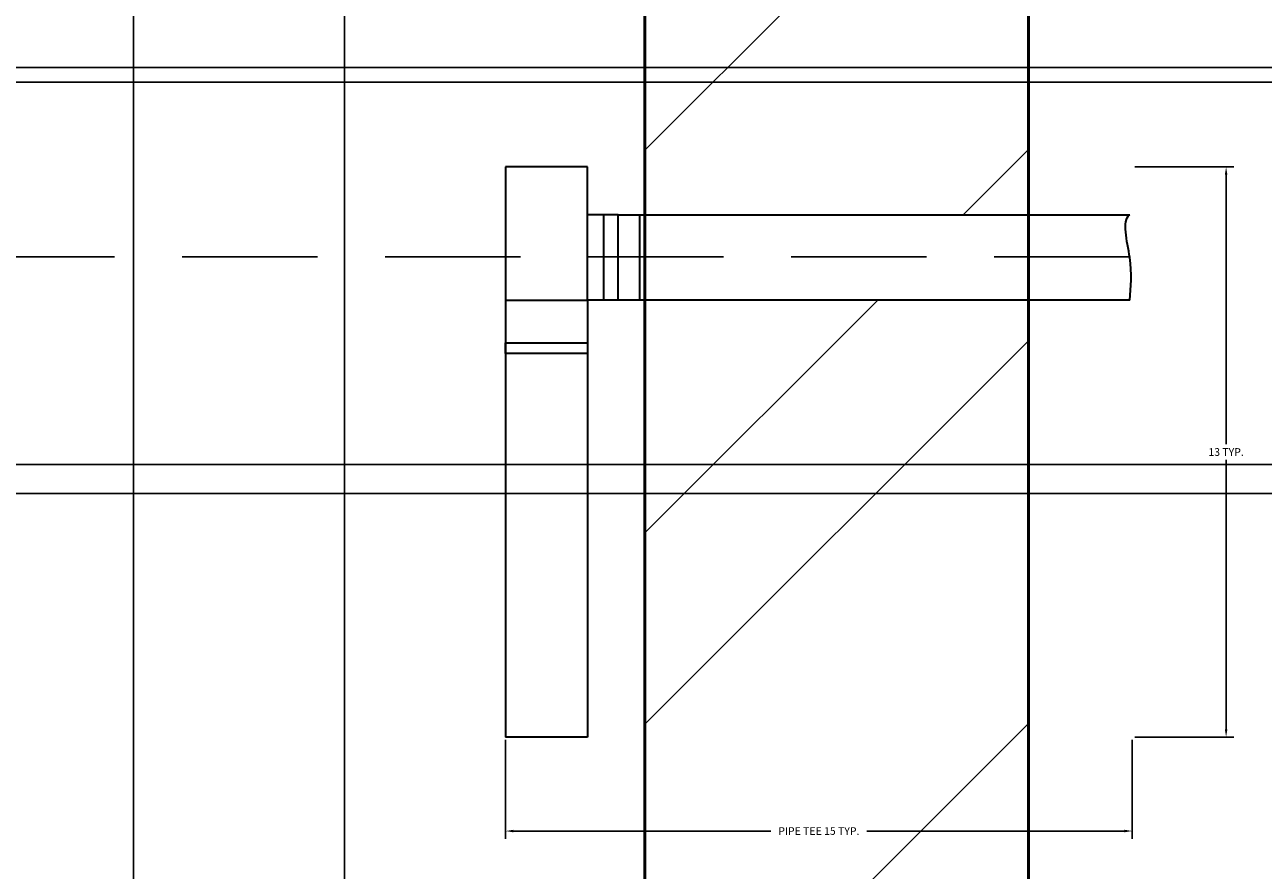
# Model space of a CAD drawing. Units: inches. Extents: x 2812 to 3051, y 1398 to 1659.
# Tile 36 of 65: x 3004 to 3033, y 1448 to 1468. Entities that reach past the tile are written whole.
import ezdxf

# ---------------------------------------------------------------- set-up
doc = ezdxf.new("R2010")
doc.units = ezdxf.units.IN
doc.linetypes.add('HIDDEN2', pattern=[4.7625, 3.175, -1.5875])
for name, color, linetype, lineweight in [('A-ANNO-DIMS', 2, 'Continuous', 18), ('P-SANR-PIPE', 4, 'Continuous', 35), ('S-CONC', 7, 'Continuous', 50), ('S-CONC-HIDN', 8, 'HIDDEN2', 25), ('S-CONC-PATT', 8, 'Continuous', 18)]:
    doc.layers.add(name, color=color, linetype=linetype, lineweight=lineweight)
doc.styles.get("Standard").update_dxf_attribs({"font": 'arial.ttf'})
doc.dimstyles.get("Standard").update_dxf_attribs({"dimtxt": 0.18, "dimasz": 0.18, "dimexe": 0.18, "dimexo": 0.0625, "dimgap": 0.09, "dimtad": 0, "dimtih": 1, "dimtoh": 1, "dimdec": 4, "dimzin": 0, "dimdsep": 46, "dimtxsty": 'Standard', "dimcen": 0.09, "dimadec": 0, "dimazin": 0, "dimtfac": 1, "dimtdec": 4, "dimtofl": 0, "dimtmove": 0, "dimatfit": 3, "dimfxl": 1, "dimtolj": 1, "dimtzin": 0, "dimarcsym": 0})

# ---------------------------------------------------------------- blocks, each defined once
blk = doc.blocks.new('PIPE-TEE-SECTION')
for p, q in [((1.921, 13.381), (0, 13.381)), ((0, 13.381), (0, 12.795)), ((1.921, 12.795), (1.921, 13.381)), ((0, 12.795), (0, 10.254)), ((1.921, 12.235), (1.921, 12.795)), ((2.641, 12.254), (1.921, 12.254)), ((1.921, 10.254), (1.921, 12.235)), ((2.299, 12.254), (2.299, 10.254)), ((2.641, 10.254), (2.641, 12.254)), ((2.641, 12.254), (14.641, 12.254)), ((2.641, 12.254), (3.141, 12.254)), ((3.141, 12.254), (3.141, 10.254)), ((0, 10.254), (1.921, 10.254)), ((0, 10.254), (0, 0)), ((2.299, 10.254), (1.921, 10.254)), ((1.921, 10.254), (1.921, 9.254)), ((14.641, 10.254), (2.299, 10.254)), ((0, 9.254), (1.921, 9.254)), ((0, 9), (0, 9.254)), ((1.921, 9.254), (1.921, 9)), ((1.921, 9), (0, 9)), ((1.921, 9), (1.921, 0)), ((1.921, 0), (0, 0))]:
    blk.add_line(p, q)
blk.add_open_spline([(14.641, 10.254), (14.669, 10.56), (14.725, 11.17), (14.444, 12.118), (14.641, 12.254)], degree=3)
blk = doc.blocks.new('*D12')
at = {"layer": 'A-ANNO-DIMS', "color": 0, "lineweight": -2, "transparency": 16777216}
for p, q in [((3015.118, 1450.968), (3015.118, 1448.646)), ((3029.815, 1450.968), (3029.815, 1448.646)), ((3015.298, 1448.826), (3021.342, 1448.826)), ((3029.635, 1448.826), (3023.591, 1448.826))]:
    blk.add_line(p, q, dxfattribs=at)
at = {"layer": 'A-ANNO-DIMS', "color": 0, "transparency": 16777216}
for points in [[(3015.298, 1448.856), (3015.298, 1448.796), (3015.118, 1448.826)], [(3029.635, 1448.856), (3029.635, 1448.796), (3029.815, 1448.826)]]:
    blk.add_solid(points, dxfattribs=at)
at = {"layer": 'Defpoints', "color": 0, "transparency": 16777216}
for p in [(3015.118, 1451.031), (3029.815, 1451.031), (3029.815, 1448.826)]:
    blk.add_point(p, dxfattribs=at)
at = {"layer": 'A-ANNO-DIMS', "color": 0, "transparency": 16777216, "insert": (3022.466, 1448.826), "char_height": 0.18, "attachment_point": 5}
blk.add_mtext('\\A1;PIPE TEE 15 TYP.', dxfattribs=at)
blk = doc.blocks.new('*D13')
at = {"layer": 'A-ANNO-DIMS', "color": 0, "lineweight": -2, "transparency": 16777216}
for p, q in [((3029.877, 1464.412), (3032.2, 1464.412)), ((3032.02, 1464.232), (3032.02, 1457.903)), ((3032.02, 1451.211), (3032.02, 1457.539)), ((3029.877, 1451.031), (3032.2, 1451.031))]:
    blk.add_line(p, q, dxfattribs=at)
at = {"layer": 'A-ANNO-DIMS', "color": 0, "transparency": 16777216}
for points in [[(3031.99, 1464.232), (3032.05, 1464.232), (3032.02, 1464.412)], [(3031.99, 1451.211), (3032.05, 1451.211), (3032.02, 1451.031)]]:
    blk.add_solid(points, dxfattribs=at)
at = {"layer": 'Defpoints', "color": 0, "transparency": 16777216}
for p in [(3029.815, 1464.412), (3032.02, 1464.412), (3029.815, 1451.031)]:
    blk.add_point(p, dxfattribs=at)
at = {"layer": 'A-ANNO-DIMS', "color": 0, "transparency": 16777216, "insert": (3032.02, 1457.721), "char_height": 0.18, "attachment_point": 5}
blk.add_mtext('\\A1;13 TYP.', dxfattribs=at)
blk = doc.blocks.new('*D33')
at = {"layer": 'A-ANNO-DIMS', "color": 0, "lineweight": -2, "transparency": 16777216}
for p, q in [((3011.337, 1597.982), (3011.337, 1397.505)), ((3018.385, 1559.757), (3018.385, 1397.505)), ((3011.517, 1397.685), (3014.468, 1397.685)), ((3018.205, 1397.685), (3015.254, 1397.685))]:
    blk.add_line(p, q, dxfattribs=at)
at = {"layer": 'A-ANNO-DIMS', "color": 0, "transparency": 16777216}
for points in [[(3011.517, 1397.715), (3011.517, 1397.655), (3011.337, 1397.685)], [(3018.205, 1397.715), (3018.205, 1397.655), (3018.385, 1397.685)]]:
    blk.add_solid(points, dxfattribs=at)
at = {"layer": 'Defpoints', "color": 0, "transparency": 16777216}
for p in [(3011.337, 1598.044), (3018.385, 1559.82), (3018.385, 1397.685)]:
    blk.add_point(p, dxfattribs=at)
at = {"layer": 'A-ANNO-DIMS', "color": 0, "transparency": 16777216, "insert": (3014.861, 1397.685), "char_height": 0.18, "attachment_point": 5}
blk.add_mtext('\\A1;7.048', dxfattribs=at)
blk = doc.blocks.new('*D34')
at = {"layer": 'A-ANNO-DIMS', "color": 0, "lineweight": -2, "transparency": 16777216}
for p, q in [((3038.462, 1593.482), (3038.462, 1397.505)), ((3027.385, 1550.757), (3027.385, 1397.505)), ((3027.565, 1397.685), (3032.468, 1397.685)), ((3038.282, 1397.685), (3033.379, 1397.685))]:
    blk.add_line(p, q, dxfattribs=at)
at = {"layer": 'A-ANNO-DIMS', "color": 0, "transparency": 16777216}
for points in [[(3027.565, 1397.715), (3027.565, 1397.655), (3027.385, 1397.685)], [(3038.282, 1397.715), (3038.282, 1397.655), (3038.462, 1397.685)]]:
    blk.add_solid(points, dxfattribs=at)
at = {"layer": 'Defpoints', "color": 0, "transparency": 16777216}
for p in [(3038.462, 1593.544), (3027.385, 1550.82), (3038.462, 1397.685)]:
    blk.add_point(p, dxfattribs=at)
at = {"layer": 'A-ANNO-DIMS', "color": 0, "transparency": 16777216, "insert": (3032.923, 1397.685), "char_height": 0.18, "attachment_point": 5}
blk.add_mtext('\\A1;11.077', dxfattribs=at)
blk = doc.blocks.new('*D47')
at = {"layer": 'A-ANNO-DIMS', "color": 0, "lineweight": -2, "transparency": 16777216}
for p, q in [((2970.385, 1487.973), (2970.385, 1397.505)), ((3006.385, 1487.973), (3006.385, 1397.505)), ((2970.565, 1397.685), (2988.166, 1397.685)), ((3006.205, 1397.685), (2988.604, 1397.685))]:
    blk.add_line(p, q, dxfattribs=at)
at = {"layer": 'A-ANNO-DIMS', "color": 0, "transparency": 16777216}
for points in [[(2970.565, 1397.715), (2970.565, 1397.655), (2970.385, 1397.685)], [(3006.205, 1397.715), (3006.205, 1397.655), (3006.385, 1397.685)]]:
    blk.add_solid(points, dxfattribs=at)
at = {"layer": 'Defpoints', "color": 0, "transparency": 16777216}
for p in [(2970.385, 1488.035), (3006.385, 1488.035), (3006.385, 1397.685)]:
    blk.add_point(p, dxfattribs=at)
at = {"layer": 'A-ANNO-DIMS', "color": 0, "transparency": 16777216, "insert": (2988.385, 1397.685), "char_height": 0.18, "attachment_point": 5}
blk.add_mtext('\\A1;36', dxfattribs=at)
blk = doc.blocks.new('*D48')
at = {"layer": 'A-ANNO-DIMS', "color": 0, "lineweight": -2, "transparency": 16777216}
for p, q in [((3006.385, 1487.973), (3006.385, 1397.505)), ((3036.385, 1409.973), (3036.385, 1397.505)), ((3006.565, 1397.685), (3021.166, 1397.685)), ((3036.205, 1397.685), (3021.603, 1397.685))]:
    blk.add_line(p, q, dxfattribs=at)
at = {"layer": 'A-ANNO-DIMS', "color": 0, "transparency": 16777216}
for points in [[(3006.565, 1397.715), (3006.565, 1397.655), (3006.385, 1397.685)], [(3036.205, 1397.715), (3036.205, 1397.655), (3036.385, 1397.685)]]:
    blk.add_solid(points, dxfattribs=at)
at = {"layer": 'Defpoints', "color": 0, "transparency": 16777216}
for p in [(3006.385, 1488.035), (3036.385, 1410.035), (3036.385, 1397.685)]:
    blk.add_point(p, dxfattribs=at)
at = {"layer": 'A-ANNO-DIMS', "color": 0, "transparency": 16777216, "insert": (3021.385, 1397.685), "char_height": 0.18, "attachment_point": 5}
blk.add_mtext('\\A1;30', dxfattribs=at)
blk = doc.blocks.new('*D67')
at = {"layer": 'A-ANNO-DIMS', "color": 0, "lineweight": -2, "transparency": 16777216}
for p, q in [((2906.065, 1457.426), (3051.178, 1457.426)), ((3050.998, 1457.246), (3050.998, 1452.608)), ((3050.998, 1447.606), (3050.998, 1452.245)), ((2914.018, 1447.426), (3051.178, 1447.426))]:
    blk.add_line(p, q, dxfattribs=at)
at = {"layer": 'A-ANNO-DIMS', "color": 0, "transparency": 16777216}
for points in [[(3050.968, 1457.246), (3051.028, 1457.246), (3050.998, 1457.426)], [(3050.968, 1447.606), (3051.028, 1447.606), (3050.998, 1447.426)]]:
    blk.add_solid(points, dxfattribs=at)
at = {"layer": 'Defpoints', "color": 0, "transparency": 16777216}
for p in [(2906.002, 1457.426), (3050.998, 1457.426), (2913.955, 1447.426)]:
    blk.add_point(p, dxfattribs=at)
at = {"layer": 'A-ANNO-DIMS', "color": 0, "transparency": 16777216, "insert": (3050.998, 1452.426), "char_height": 0.18, "attachment_point": 5}
blk.add_mtext('\\A1;10', dxfattribs=at)
blk = doc.blocks.new('*D68')
at = {"layer": 'A-ANNO-DIMS', "color": 0, "lineweight": -2, "transparency": 16777216}
for p, q in [((2898.12, 1466.402), (3051.178, 1466.402)), ((3050.998, 1466.222), (3050.998, 1462.096)), ((3050.998, 1457.606), (3050.998, 1461.733)), ((2906.065, 1457.426), (3051.178, 1457.426))]:
    blk.add_line(p, q, dxfattribs=at)
at = {"layer": 'A-ANNO-DIMS', "color": 0, "transparency": 16777216}
for points in [[(3050.968, 1466.222), (3051.028, 1466.222), (3050.998, 1466.402)], [(3050.968, 1457.606), (3051.028, 1457.606), (3050.998, 1457.426)]]:
    blk.add_solid(points, dxfattribs=at)
at = {"layer": 'Defpoints', "color": 0, "transparency": 16777216}
for p in [(2898.058, 1466.402), (3050.998, 1466.402), (2906.002, 1457.426)]:
    blk.add_point(p, dxfattribs=at)
at = {"layer": 'A-ANNO-DIMS', "color": 0, "transparency": 16777216, "insert": (3050.998, 1461.914), "char_height": 0.18, "attachment_point": 5}
blk.add_mtext('\\A1;8.976', dxfattribs=at)
blk = doc.blocks.new('*D81')
at = {"layer": 'A-ANNO-DIMS', "color": 0, "lineweight": -2, "transparency": 16777216}
for p, q in [((2988.31, 1456.747), (3051.178, 1456.747)), ((3050.998, 1456.567), (3050.998, 1451.929)), ((3050.998, 1446.927), (3050.998, 1451.565)), ((2996.018, 1446.747), (3051.178, 1446.747))]:
    blk.add_line(p, q, dxfattribs=at)
at = {"layer": 'A-ANNO-DIMS', "color": 0, "transparency": 16777216}
for points in [[(3050.968, 1456.567), (3051.028, 1456.567), (3050.998, 1456.747)], [(3050.968, 1446.927), (3051.028, 1446.927), (3050.998, 1446.747)]]:
    blk.add_solid(points, dxfattribs=at)
at = {"layer": 'Defpoints', "color": 0, "transparency": 16777216}
for p in [(2988.248, 1456.747), (3050.998, 1456.747), (2995.956, 1446.747)]:
    blk.add_point(p, dxfattribs=at)
at = {"layer": 'A-ANNO-DIMS', "color": 0, "transparency": 16777216, "insert": (3050.998, 1451.747), "char_height": 0.18, "attachment_point": 5}
blk.add_mtext('\\A1;10', dxfattribs=at)
blk = doc.blocks.new('*D82')
at = {"layer": 'A-ANNO-DIMS', "color": 0, "lineweight": -2, "transparency": 16777216}
for p, q in [((2978.018, 1466.747), (3051.178, 1466.747)), ((3050.998, 1466.567), (3050.998, 1461.929)), ((3050.998, 1456.927), (3050.998, 1461.565)), ((2988.31, 1456.747), (3051.178, 1456.747))]:
    blk.add_line(p, q, dxfattribs=at)
at = {"layer": 'A-ANNO-DIMS', "color": 0, "transparency": 16777216}
for points in [[(3050.968, 1466.567), (3051.028, 1466.567), (3050.998, 1466.747)], [(3050.968, 1456.927), (3051.028, 1456.927), (3050.998, 1456.747)]]:
    blk.add_solid(points, dxfattribs=at)
at = {"layer": 'Defpoints', "color": 0, "transparency": 16777216}
for p in [(2977.956, 1466.747), (3050.998, 1466.747), (2988.248, 1456.747)]:
    blk.add_point(p, dxfattribs=at)
at = {"layer": 'A-ANNO-DIMS', "color": 0, "transparency": 16777216, "insert": (3050.998, 1461.747), "char_height": 0.18, "attachment_point": 5}
blk.add_mtext('\\A1;10', dxfattribs=at)

msp = doc.modelspace()

# ---------------------------------------------------------------- hatches: boundary and pattern name
at = {"layer": 'S-CONC-PATT'}
h = msp.add_hatch(dxfattribs=at)
h.set_pattern_fill('ANSI32', color=256)
h.paths.add_polyline_path([(3027.3849, 1646.82), (2835.3849, 1646.82), (2835.3849, 1603.2296), (2844.3849, 1603.2296), (2844.3849, 1637.82), (3018.3849, 1637.82), (3018.3849, 1602.5441), (3027.3849, 1602.5441)])
h.paths.add_polyline_path([(2844.3849, 1594.2296), (2835.3849, 1594.2296), (2835.3849, 1550.82), (3027.3849, 1550.82), (3027.3849, 1593.5441), (3018.3849, 1593.5441), (3018.3849, 1559.82), (2844.3849, 1559.82)])
h.paths.add_polyline_path([(2844.3849, 1482.0354), (2835.3849, 1482.0354), (2835.3849, 1463.4959), (2844.3849, 1463.4959)])
h.paths.add_polyline_path([(2844.3849, 1461.4959), (2835.3849, 1461.4959), (2835.3849, 1416.0354), (2844.3849, 1416.0354)])
h.paths.add_polyline_path([(3027.3849, 1482.0354), (3018.3849, 1482.0354), (3018.3849, 1463.2854), (3027.3849, 1463.2854)])
h.paths.add_polyline_path([(3027.3849, 1461.2854), (3018.3849, 1461.2854), (3018.3849, 1416.0354), (3027.3849, 1416.0354)])
h.paths.add_polyline_path([(2961.3849, 1448.4738), (2952.3849, 1448.4738), (2952.3849, 1416.0354), (2961.3849, 1416.0354)])
h.paths.add_polyline_path([(2961.3849, 1462.3026), (2952.3849, 1462.3026), (2952.3849, 1450.4738), (2961.3849, 1450.4738)])
h.paths.add_polyline_path([(2961.3849, 1472.0354), (2952.3849, 1472.0354), (2952.3849, 1462.3026), (2961.3849, 1462.3026)])

# ---------------------------------------------------------------- linework, layer by layer
at = {"layer": 'S-CONC'}
for p, q in [((3018.3849, 1482.0354), (3018.3849, 1416.0354)), ((3027.3849, 1482.0354), (3027.3849, 1416.0354))]:
    msp.add_line(p, q, dxfattribs=at)
at = {"layer": 'S-CONC-HIDN'}
msp.add_line((3029.7562, 1462.3026), (2835.3849, 1462.3026), dxfattribs=at)

# ---------------------------------------------------------------- block references
at = {"layer": 'P-SANR-PIPE'}
msp.add_blockref('PIPE-TEE-SECTION', (3015.118, 1451.031), dxfattribs=at)

# ---------------------------------------------------------------- dimensions: what is measured, and where the dimension line sits
at = {"layer": 'A-ANNO-DIMS'}
for base, p1, p2, override, picture, middle in [((3018.3849, 1397.6854), (3011.3373, 1598.0441), (3018.3849, 1559.82), {"dimdec": 3, "dimlfac": 1, "dimrnd": 0, "dimzin": 0, "dimdsep": 46, "dimlunit": 2}, '*D33', (3014.8611, 1397.6854)), ((3038.4621, 1397.6854), (3027.3849, 1550.82), (3038.4621, 1593.5441), {"dimdec": 3, "dimlfac": 1, "dimrnd": 0, "dimzin": 0, "dimdsep": 46, "dimlunit": 2}, '*D34', (3032.9235, 1397.6854)), ((3006.3849, 1397.6854), (2970.3849, 1488.0354), (3006.3849, 1488.0354), {"dimdec": 0, "dimlfac": 1, "dimrnd": 0, "dimzin": 0, "dimdsep": 46, "dimlunit": 2}, '*D47', (2988.3849, 1397.6854)), ((3036.3849, 1397.6854), (3006.3849, 1488.0354), (3036.3849, 1410.0354), {"dimdec": 0, "dimlfac": 1, "dimrnd": 0, "dimzin": 0, "dimdsep": 46, "dimlunit": 2}, '*D48', (3021.3849, 1397.6854))]:
    dim = msp.add_linear_dim(base=base, p1=p1, p2=p2, dimstyle='Standard', override=override, dxfattribs=at)
    dim.commit()
    dim.dimension.update_dxf_attribs({"geometry": picture, "text_midpoint": middle})
for base, p1, p2, override, picture, middle in [((3050.998, 1466.7474), (2988.2478, 1456.7474), (2977.9558, 1466.7474), {"dimdec": 0, "dimlfac": 1, "dimrnd": 0, "dimzin": 0, "dimdsep": 46, "dimlunit": 2}, '*D82', (3050.998, 1461.7474)), ((3050.998, 1466.4024), (2906.0021, 1457.4265), (2898.0577, 1466.4024), {"dimdec": 3, "dimlfac": 1, "dimrnd": 0, "dimzin": 0, "dimdsep": 46, "dimlunit": 2}, '*D68', (3050.998, 1461.9144)), ((3050.998, 1457.4265), (2913.9551, 1447.4265), (2906.0021, 1457.4265), {"dimdec": 0, "dimlfac": 1, "dimrnd": 0, "dimzin": 0, "dimdsep": 46, "dimlunit": 2}, '*D67', (3050.998, 1452.4265)), ((3050.998, 1456.7474), (2995.9558, 1446.7474), (2988.2478, 1456.7474), {"dimdec": 0, "dimlfac": 1, "dimrnd": 0, "dimzin": 0, "dimdsep": 46, "dimlunit": 2}, '*D81', (3050.998, 1451.7474))]:
    dim = msp.add_linear_dim(base=base, p1=p1, p2=p2, angle=90, dimstyle='Standard', override=override, dxfattribs=at)
    dim.commit()
    dim.dimension.update_dxf_attribs({"geometry": picture, "text_midpoint": middle})
dim = msp.add_linear_dim(base=(3032.0196, 1464.4116), p1=(3029.815, 1451.0307), p2=(3029.815, 1464.4116), angle=90, text='<> TYP.', dimstyle='Standard', override={"dimdec": 0, "dimlfac": 1, "dimrnd": 0, "dimzin": 0, "dimdsep": 46, "dimlunit": 2}, dxfattribs=at)
dim.commit()
dim.dimension.update_dxf_attribs({"geometry": '*D13', "text_midpoint": (3032.0196, 1457.7211)})
dim = msp.add_linear_dim(base=(3029.815, 1448.8261), p1=(3015.1177, 1451.0307), p2=(3029.815, 1451.0307), text='PIPE TEE <> TYP.', dimstyle='Standard', override={"dimdec": 0, "dimlfac": 1, "dimrnd": 0, "dimzin": 0, "dimdsep": 46, "dimlunit": 2}, dxfattribs=at)
dim.commit()
dim.dimension.update_dxf_attribs({"geometry": '*D12', "text_midpoint": (3022.4664, 1448.8261)})

doc.saveas('drawing.dxf')
